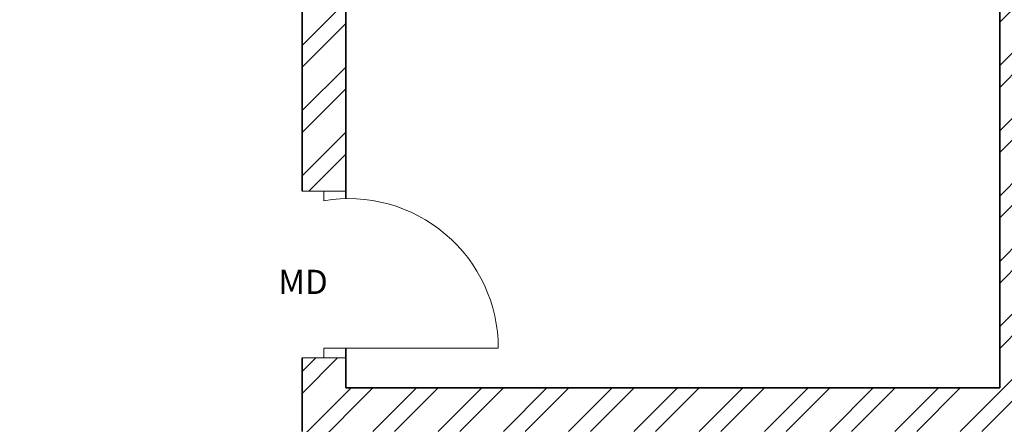
# Model space of a CAD drawing. Units: inches. Extents: x 2120 to 4013, y 1390 to 3019.
# Tile 35 of 59: x 2657 to 2861, y 1964 to 2048. Entities that reach past the tile are written whole.
import ezdxf

# ---------------------------------------------------------------- set-up
doc = ezdxf.new("R2010")
doc.units = ezdxf.units.IN
for name, color, linetype, lineweight in [('A-ANNO-TEXT', 7, 'Continuous', 18), ('A-DOOR', 3, 'Continuous', 18), ('A-WALL', 7, 'Continuous', 35), ('A-WALL-PATT', 252, 'Continuous', 13)]:
    doc.layers.add(name, color=color, linetype=linetype, lineweight=lineweight)
doc.styles.get("Standard").update_dxf_attribs({"font": 'arial.ttf'})

msp = doc.modelspace()

# ---------------------------------------------------------------- hatches: boundary and pattern name
at = {"layer": 'A-WALL-PATT'}
h = msp.add_hatch(dxfattribs=at)
h.set_pattern_fill('ANSI32', color=256)
h.paths.add_polyline_path([(2271.7331, 2343.531), (2283.3788, 2343.531), (2283.3788, 2348.031), (2283.3788, 2352.5306), (2262.7331, 2352.5306), (2262.7331, 2182.638), (2267.2331, 2182.638), (2271.7331, 2182.638), (2271.7331, 2219.031), (2391.7331, 2219.031), (2391.7331, 2214.189), (2393.9831, 2214.189), (2396.2331, 2214.189), (2396.2331, 2219.031), (2420.2331, 2219.031), (2420.2331, 2225.7535), (2417.2197, 2225.7535), (2415.7331, 2225.7535), (2415.7331, 2223.5306), (2271.7331, 2223.5306)])
h.paths.add_polyline_path([(2380.0942, 2352.5306), (2343.3788, 2352.5306), (2343.3788, 2343.531), (2363.2331, 2343.531), (2363.2331, 2288.8489), (2365.4831, 2288.8489), (2367.7331, 2288.8489), (2367.7331, 2343.531), (2380.0942, 2343.531)], flags=17)
h.paths.add_polyline_path([(2432.4339, 2352.5306), (2404.0943, 2352.5306), (2404.0943, 2343.531), (2415.7331, 2343.531), (2415.7331, 2264.0306), (2367.7331, 2264.0306), (2367.7331, 2266.4872), (2363.2331, 2266.4872), (2363.2331, 2259.531), (2367.7331, 2259.531), (2415.7331, 2259.531), (2415.7331, 2255.0658), (2420.2331, 2255.0658), (2420.2331, 2259.531), (2424.5717, 2259.531), (2424.5717, 2261.781), (2424.5717, 2264.0306), (2420.2331, 2264.0306), (2420.2331, 2343.531), (2432.4339, 2343.531)])
h.paths.add_polyline_path([(2508.9115, 2352.5306), (2456.4339, 2352.5306), (2456.4339, 2343.531), (2468.2331, 2343.531), (2468.2331, 2264.0306), (2448.0487, 2264.0306), (2448.0487, 2259.531), (2468.2331, 2259.531), (2468.2331, 2255.5496), (2472.7331, 2255.5496), (2472.7331, 2343.531), (2508.9115, 2343.531)])
h.paths.add_polyline_path([(2637.7331, 2352.5306), (2544.9116, 2352.5306), (2544.9116, 2343.531), (2589.7331, 2343.531), (2633.2331, 2343.531), (2637.7331, 2343.531)])
h.paths.add_polyline_path([(2594.2331, 2343.5306), (2589.7331, 2343.5306), (2589.7331, 2259.5306), (2589.7331, 2252.4915), (2591.9831, 2252.4915), (2594.2331, 2252.4915)])
h.paths.add_polyline_path([(2637.7331, 2223.5306), (2594.2331, 2223.5306), (2594.2331, 2230.1988), (2591.9831, 2230.1988), (2589.7331, 2230.1988), (2589.7331, 2223.5306), (2472.7331, 2223.5306), (2468.2331, 2223.5306), (2468.2331, 2219.031), (2628.7331, 2219.031), (2628.7331, 2138.031), (2637.7331, 2138.031)])
h.paths.add_polyline_path([(3822.6535, 2458.4402), (3874.9468, 2458.4402), (3874.9468, 2476.9866), (3822.6535, 2476.9866)], flags=9)
h.paths.add_polyline_path([(3834.6921, 2781.8174), (3935.9206, 2781.8174), (3935.9206, 2800.3638), (3834.6921, 2800.3638)], flags=9)
h.paths.add_polyline_path([(3832.2843, 2837.9683), (3884.5776, 2837.9683), (3884.5776, 2856.5146), (3832.2843, 2856.5146)], flags=9)
h.paths.add_polyline_path([(3830.9388, 2861.4782), (3956.8958, 2861.4782), (3956.8958, 2880.0245), (3830.9388, 2880.0245)], flags=9)
h.paths.add_polyline_path([(3870.6966, 2352.5752), (3887.9272, 2352.5752), (3887.9272, 2377.3037), (3870.6966, 2377.3037)], flags=9)
h.paths.add_polyline_path([(3289.2701, 2413.161), (3435.2223, 2413.161), (3435.2223, 2450.2538), (3289.2701, 2450.2538)], flags=9)
h.paths.add_polyline_path([(2487.6944, 2414.3601), (2637.8335, 2414.3601), (2637.8335, 2451.4528), (2487.6944, 2451.4528)], flags=9)
h.paths.add_polyline_path([(2567.3724, 1457.9199), (2815.296, 1457.9199), (2815.296, 1495.0127), (2567.3724, 1495.0127)], flags=9)
h.paths.add_polyline_path([(2655.3825, 2093.2363), (2685.9555, 2093.2363), (2685.9555, 2111.8937), (2655.3825, 2111.8937)], flags=9)
h.paths.add_polyline_path([(2543.9218, 1550.6671), (2587.8406, 1550.6671), (2587.8406, 1569.3244), (2543.9218, 1569.3244)], flags=9)
h.paths.add_polyline_path([(2905.1384, 1543.8113), (2949.0572, 1543.8113), (2949.0572, 1562.4686), (2905.1384, 1562.4686)], flags=9)
h.paths.add_polyline_path([(2736.4118, 1702.4736), (2784.2153, 1702.4736), (2784.2153, 1721.1309), (2736.4118, 1721.1309)], flags=9)
h.paths.add_polyline_path([(2912.8666, 1710.4168), (2951.707, 1710.4168), (2951.707, 1729.0741), (2912.8666, 1729.0741)], flags=9)
h.paths.add_polyline_path([(2923.5785, 1763.5038), (2959.7279, 1763.5038), (2959.7279, 1782.1611), (2923.5785, 1782.1611)], flags=9)
h.paths.add_polyline_path([(2925.2114, 1809.6137), (2967.1861, 1809.6137), (2967.1861, 1828.271), (2925.2114, 1828.271)], flags=9)
h.paths.add_polyline_path([(2996.2711, 1878.9003), (2996.2711, 1913.109), (2977.6138, 1913.109), (2977.6138, 1878.9003)], flags=9)
h.paths.add_polyline_path([(2883.0859, 1895.7192), (2927.1855, 1895.7192), (2927.1855, 1914.3766), (2883.0859, 1914.3766)], flags=9)
h.paths.add_polyline_path([(2787.3924, 1810.8013), (2841.0213, 1810.8013), (2841.0213, 1829.4587), (2787.3924, 1829.4587)], flags=9)
h.paths.add_polyline_path([(2775.6399, 2101.7395), (2829.2689, 2101.7395), (2829.2689, 2120.3968), (2775.6399, 2120.3968)], flags=9)
h.paths.add_polyline_path([(2913.0263, 2075.817), (2951.8667, 2075.817), (2951.8667, 2094.4744), (2913.0263, 2094.4744)], flags=9)
h.paths.add_polyline_path([(2929.966, 2133.3669), (2966.1154, 2133.3669), (2966.1154, 2152.0243), (2929.966, 2152.0243)], flags=9)
h.paths.add_polyline_path([(2932.7502, 2182.6088), (2968.8996, 2182.6088), (2968.8996, 2201.2662), (2932.7502, 2201.2662)], flags=9)
h.paths.add_polyline_path([(2996.0681, 2266.3173), (2996.0681, 2300.5261), (2977.4108, 2300.5261), (2977.4108, 2266.3173)], flags=9)
h.paths.add_polyline_path([(2885.1039, 2279.2186), (2929.2035, 2279.2186), (2929.2035, 2297.8759), (2885.1039, 2297.8759)], flags=9)
h.paths.add_polyline_path([(2735.7042, 2218.3197), (2783.5078, 2218.3197), (2783.5078, 2236.9771), (2735.7042, 2236.9771)], flags=9)
h.paths.add_polyline_path([(2635.6049, 2044.0085), (2648.9678, 2044.0085), (2648.9678, 2054.312), (2635.6049, 2054.312)], flags=9)
h.paths.add_polyline_path([(2714.0148, 1923.0473), (2727.3777, 1923.0473), (2727.3777, 1933.3508), (2714.0148, 1933.3508)], flags=9)
h.paths.add_polyline_path([(2709.0345, 1988.1628), (2722.3974, 1988.1628), (2722.3974, 1998.4663), (2709.0345, 1998.4663)], flags=9)
h.paths.add_polyline_path([(2592.8935, 1962.1763), (2606.2564, 1962.1763), (2606.2564, 1972.4799), (2592.8935, 1972.4799)], flags=9)
h.paths.add_polyline_path([(2618.3996, 1985.9724), (2644.1942, 1985.9724), (2644.1942, 1996.2759), (2618.3996, 1996.2759)], flags=9)
h.paths.add_polyline_path([(2601.279, 1920.5869), (2614.6419, 1920.5869), (2614.6419, 1930.8904), (2601.279, 1930.8904)], flags=9)
h.paths.add_polyline_path([(2692.3278, 1932.7645), (2704.5311, 1932.7645), (2704.5311, 1943.0681), (2692.3278, 1943.0681)], flags=9)
h.paths.add_polyline_path([(2311.122, 1672.7318), (2355.0408, 1672.7318), (2355.0408, 1691.3892), (2311.122, 1691.3892)], flags=9)
h.paths.add_polyline_path([(2456.2551, 1632.3198), (2492.4796, 1632.3198), (2492.4796, 1650.9772), (2456.2551, 1650.9772)], flags=9)
h.paths.add_polyline_path([(2401.0766, 1631.4793), (2437.301, 1631.4793), (2437.301, 1650.1367), (2401.0766, 1650.1367)], flags=9)
h.paths.add_polyline_path([(2546.7054, 1700.9235), (2594.509, 1700.9235), (2594.509, 1719.5809), (2546.7054, 1719.5809)], flags=9)
h.paths.add_polyline_path([(2445.4866, 1766.9937), (2497.5261, 1766.9937), (2497.5261, 1785.651), (2445.4866, 1785.651)], flags=9)
h.paths.add_polyline_path([(2287.9992, 1739.7675), (2326.8396, 1739.7675), (2326.8396, 1758.4248), (2287.9992, 1758.4248)], flags=9)
h.paths.add_polyline_path([(2458.5279, 1924.7607), (2510.5675, 1924.7607), (2510.5675, 1943.4181), (2458.5279, 1943.4181)], flags=9)
h.paths.add_polyline_path([(2309.2811, 1902.7642), (2345.4305, 1902.7642), (2345.4305, 1921.4215), (2309.2811, 1921.4215)], flags=9)
h.paths.add_polyline_path([(2490.7554, 2018.9392), (2530.7896, 2018.9392), (2530.7896, 2037.5965), (2490.7554, 2037.5965)], flags=9)
h.paths.add_polyline_path([(2402.143, 2024.7393), (2438.5414, 2024.7393), (2438.5414, 2043.3966), (2402.143, 2043.3966)], flags=9)
h.paths.add_polyline_path([(2287.856, 1931.7926), (2326.6964, 1931.7926), (2326.6964, 1950.4499), (2287.856, 1950.4499)], flags=9)
h.paths.add_polyline_path([(2281.7979, 2193.5771), (2320.6383, 2193.5771), (2320.6383, 2212.2344), (2281.7979, 2212.2344)], flags=25)
h.paths.add_polyline_path([(2484.0754, 2093.892), (2536.115, 2093.892), (2536.115, 2112.5494), (2484.0754, 2112.5494)], flags=9)
h.paths.add_polyline_path([(2624.7948, 2281.8639), (2624.7948, 2311.4137), (2606.1375, 2311.4137), (2606.1375, 2281.8639)], flags=9)
h.paths.add_polyline_path([(2507.5036, 2290.3639), (2541.934, 2290.3639), (2541.934, 2309.0212), (2507.5036, 2309.0212)], flags=9)
h.paths.add_polyline_path([(2423.1076, 2285.2202), (2459.332, 2285.2202), (2459.332, 2303.8776), (2423.1076, 2303.8776)], flags=9)
h.paths.add_polyline_path([(2374.5467, 2289.6272), (2410.7711, 2289.6272), (2410.7711, 2308.2846), (2374.5467, 2308.2846)], flags=25)
h.paths.add_polyline_path([(2277.4907, 2227.5651), (2316.3311, 2227.5651), (2316.3311, 2246.2224), (2277.4907, 2246.2224)], flags=25)
h.paths.add_polyline_path([(2655.3825, 2093.2367), (2685.9555, 2093.2367), (2685.9555, 2111.894), (2655.3825, 2111.894)], flags=9)
h.paths.add_polyline_path([(2543.9217, 1550.6674), (2587.8406, 1550.6674), (2587.8406, 1569.3247), (2543.9217, 1569.3247)], flags=9)
h.paths.add_polyline_path([(2905.1384, 1543.8116), (2949.0572, 1543.8116), (2949.0572, 1562.4689), (2905.1384, 1562.4689)], flags=9)
h.paths.add_polyline_path([(2736.4118, 1702.4739), (2784.2153, 1702.4739), (2784.2153, 1721.1312), (2736.4118, 1721.1312)], flags=9)
h.paths.add_polyline_path([(2912.8666, 1710.4171), (2951.707, 1710.4171), (2951.707, 1729.0744), (2912.8666, 1729.0744)], flags=9)
h.paths.add_polyline_path([(2923.5785, 1763.5041), (2959.7279, 1763.5041), (2959.7279, 1782.1614), (2923.5785, 1782.1614)], flags=9)
h.paths.add_polyline_path([(2925.2114, 1809.614), (2967.1861, 1809.614), (2967.1861, 1828.2713), (2925.2114, 1828.2713)], flags=9)
h.paths.add_polyline_path([(2996.2711, 1878.9006), (2996.2711, 1913.1094), (2977.6137, 1913.1094), (2977.6137, 1878.9006)], flags=9)
h.paths.add_polyline_path([(2883.0859, 1895.7195), (2927.1855, 1895.7195), (2927.1855, 1914.3769), (2883.0859, 1914.3769)], flags=9)
h.paths.add_polyline_path([(2787.3924, 1810.8016), (2841.0213, 1810.8016), (2841.0213, 1829.459), (2787.3924, 1829.459)], flags=9)
h.paths.add_polyline_path([(2775.6399, 2101.7398), (2829.2688, 2101.7398), (2829.2688, 2120.3971), (2775.6399, 2120.3971)], flags=9)
h.paths.add_polyline_path([(2913.0263, 2075.8173), (2951.8667, 2075.8173), (2951.8667, 2094.4747), (2913.0263, 2094.4747)], flags=9)
h.paths.add_polyline_path([(2929.966, 2133.3672), (2966.1154, 2133.3672), (2966.1154, 2152.0246), (2929.966, 2152.0246)], flags=9)
h.paths.add_polyline_path([(2932.7502, 2182.6091), (2968.8996, 2182.6091), (2968.8996, 2201.2665), (2932.7502, 2201.2665)], flags=9)
h.paths.add_polyline_path([(2996.0681, 2266.3176), (2996.0681, 2300.5264), (2977.4108, 2300.5264), (2977.4108, 2266.3176)], flags=9)
h.paths.add_polyline_path([(2885.1039, 2279.2189), (2929.2035, 2279.2189), (2929.2035, 2297.8762), (2885.1039, 2297.8762)], flags=9)
h.paths.add_polyline_path([(2735.7042, 2218.32), (2783.5078, 2218.32), (2783.5078, 2236.9774), (2735.7042, 2236.9774)], flags=9)
h.paths.add_polyline_path([(2635.6048, 2044.0088), (2648.9677, 2044.0088), (2648.9677, 2054.3123), (2635.6048, 2054.3123)], flags=9)
h.paths.add_polyline_path([(2714.0148, 1923.0476), (2727.3777, 1923.0476), (2727.3777, 1933.3511), (2714.0148, 1933.3511)], flags=9)
h.paths.add_polyline_path([(2709.0345, 1988.1631), (2722.3974, 1988.1631), (2722.3974, 1998.4666), (2709.0345, 1998.4666)], flags=9)
h.paths.add_polyline_path([(2592.8935, 1962.1766), (2606.2564, 1962.1766), (2606.2564, 1972.4802), (2592.8935, 1972.4802)], flags=9)
h.paths.add_polyline_path([(2618.3995, 1985.9727), (2644.1942, 1985.9727), (2644.1942, 1996.2762), (2618.3995, 1996.2762)], flags=9)
h.paths.add_polyline_path([(2601.279, 1920.5872), (2614.6419, 1920.5872), (2614.6419, 1930.8908), (2601.279, 1930.8908)], flags=9)
h.paths.add_polyline_path([(2692.3278, 1932.7648), (2704.5311, 1932.7648), (2704.5311, 1943.0684), (2692.3278, 1943.0684)], flags=9)
h.paths.add_polyline_path([(2311.122, 1672.7321), (2355.0408, 1672.7321), (2355.0408, 1691.3895), (2311.122, 1691.3895)], flags=9)
h.paths.add_polyline_path([(2456.2551, 1632.3201), (2492.4795, 1632.3201), (2492.4795, 1650.9775), (2456.2551, 1650.9775)], flags=9)
h.paths.add_polyline_path([(2401.0766, 1631.4796), (2437.301, 1631.4796), (2437.301, 1650.137), (2401.0766, 1650.137)], flags=9)
h.paths.add_polyline_path([(2546.7054, 1700.9238), (2594.509, 1700.9238), (2594.509, 1719.5812), (2546.7054, 1719.5812)], flags=9)
h.paths.add_polyline_path([(2445.4866, 1766.994), (2497.5261, 1766.994), (2497.5261, 1785.6513), (2445.4866, 1785.6513)], flags=9)
h.paths.add_polyline_path([(2287.9992, 1739.7678), (2326.8396, 1739.7678), (2326.8396, 1758.4251), (2287.9992, 1758.4251)], flags=9)
h.paths.add_polyline_path([(2458.5279, 1924.7611), (2510.5675, 1924.7611), (2510.5675, 1943.4184), (2458.5279, 1943.4184)], flags=9)
h.paths.add_polyline_path([(2309.2811, 1902.7645), (2345.4305, 1902.7645), (2345.4305, 1921.4218), (2309.2811, 1921.4218)], flags=9)
h.paths.add_polyline_path([(2490.7554, 2018.9395), (2530.7895, 2018.9395), (2530.7895, 2037.5968), (2490.7554, 2037.5968)], flags=9)
h.paths.add_polyline_path([(2402.143, 2024.7396), (2438.5413, 2024.7396), (2438.5413, 2043.3969), (2402.143, 2043.3969)], flags=9)
h.paths.add_polyline_path([(2287.856, 1931.7929), (2326.6964, 1931.7929), (2326.6964, 1950.4502), (2287.856, 1950.4502)], flags=9)
h.paths.add_polyline_path([(2281.7979, 2193.5774), (2320.6383, 2193.5774), (2320.6383, 2212.2347), (2281.7979, 2212.2347)], flags=25)
h.paths.add_polyline_path([(2484.0754, 2093.8924), (2536.115, 2093.8924), (2536.115, 2112.5497), (2484.0754, 2112.5497)], flags=9)
h.paths.add_polyline_path([(2624.7948, 2281.8642), (2624.7948, 2311.414), (2606.1374, 2311.414), (2606.1374, 2281.8642)], flags=9)
h.paths.add_polyline_path([(2507.5035, 2290.3642), (2541.934, 2290.3642), (2541.934, 2309.0215), (2507.5035, 2309.0215)], flags=9)
h.paths.add_polyline_path([(2423.1075, 2285.2205), (2459.332, 2285.2205), (2459.332, 2303.8779), (2423.1075, 2303.8779)], flags=9)
h.paths.add_polyline_path([(2374.5467, 2289.6275), (2410.7711, 2289.6275), (2410.7711, 2308.2849), (2374.5467, 2308.2849)], flags=25)
h.paths.add_polyline_path([(2277.4907, 2227.5654), (2316.3311, 2227.5654), (2316.3311, 2246.2227), (2277.4907, 2246.2227)], flags=25)
h = msp.add_hatch(dxfattribs=at)
h.set_pattern_fill('ANSI32', color=256)
h.paths.add_polyline_path([(2271.7331, 1980.389), (2262.7331, 1980.389), (2262.7331, 1912.8434), (2267.2331, 1912.8434), (2271.7331, 1912.8434), (2271.7331, 1922.531), (2351.2331, 1922.531), (2351.2331, 1901.4728), (2355.7331, 1901.4728), (2355.7331, 1922.531), (2357.9815, 1922.531), (2357.9815, 1926.5306), (2271.7331, 1926.5306)])
h.paths.add_polyline_path([(2589.2331, 1949.1622), (2584.7331, 1949.1622), (2580.2331, 1949.1622), (2580.2331, 1874.5306), (2355.7331, 1874.5306), (2355.7331, 1880.1922), (2351.2331, 1880.1922), (2351.2331, 1874.5306), (2271.7331, 1874.5306), (2271.7331, 1888.8431), (2262.7331, 1888.8431), (2262.7331, 1842.2909), (2267.2331, 1842.2909), (2271.7331, 1842.2909), (2271.7331, 1865.531), (2415.7331, 1865.531), (2415.7331, 1779.7286), (2420.2331, 1779.7286), (2420.2331, 1865.531), (2589.2331, 1865.531)])
h.paths.add_polyline_path([(2271.7331, 1782.2906), (2262.7331, 1782.2906), (2262.7331, 1711.4639), (2267.2331, 1711.4639), (2271.7331, 1711.4639), (2271.7331, 1738.031), (2420.2331, 1738.031), (2420.2331, 1742.531), (2420.2331, 1747.3376), (2417.9831, 1747.3376), (2415.7331, 1747.3376), (2415.7331, 1742.5306), (2271.7331, 1742.5306)])
h.paths.add_polyline_path([(2271.7331, 1627.031), (2362.3957, 1627.031), (2362.3957, 1629.281), (2362.3957, 1631.5306), (2271.7331, 1631.5306), (2271.7331, 1675.4636), (2262.7331, 1675.4636), (2262.7331, 1581.531), (2405.3032, 1581.531), (2405.3032, 1586.031), (2405.3032, 1590.5306), (2396.2331, 1590.5306), (2396.2331, 1691.4513), (2418.7206, 1691.4513), (2418.7206, 1695.951), (2396.2331, 1695.951), (2391.7331, 1695.951), (2391.7331, 1631.5306), (2386.7425, 1631.5306), (2386.7425, 1629.2806), (2386.7425, 1627.031), (2391.7331, 1627.031), (2391.7331, 1586.1709), (2271.7331, 1586.1709)])
h.paths.add_polyline_path([(2459.6703, 1590.5306), (2429.3032, 1590.5306), (2429.3032, 1581.531), (2459.6703, 1581.531), (2459.6703, 1586.031)])
h.paths.add_polyline_path([(2501.2331, 1590.531), (2501.2331, 1665.0195), (2498.9831, 1665.0195), (2496.7331, 1665.0195), (2496.7331, 1590.5306), (2483.8201, 1590.5306), (2483.8201, 1590.1579), (2483.6704, 1590.1579), (2483.6704, 1581.531), (2505.0196, 1581.531), (2505.0196, 1583.781), (2505.0196, 1586.0306), (2501.2331, 1586.0306)])
h.paths.add_polyline_path([(2544.1361, 1583.781), (2544.1361, 1586.0306), (2527.1368, 1586.0306), (2527.1368, 1583.7806), (2527.1368, 1581.531), (2544.1361, 1581.531)])
h.paths.add_polyline_path([(3822.6535, 2458.4402), (3874.9468, 2458.4402), (3874.9468, 2476.9866), (3822.6535, 2476.9866)], flags=9)
h.paths.add_polyline_path([(3834.6921, 2781.8174), (3935.9206, 2781.8174), (3935.9206, 2800.3638), (3834.6921, 2800.3638)], flags=9)
h.paths.add_polyline_path([(3832.2843, 2837.9683), (3884.5776, 2837.9683), (3884.5776, 2856.5146), (3832.2843, 2856.5146)], flags=9)
h.paths.add_polyline_path([(3830.9388, 2861.4782), (3956.8958, 2861.4782), (3956.8958, 2880.0245), (3830.9388, 2880.0245)], flags=9)
h.paths.add_polyline_path([(3870.6966, 2352.5752), (3887.9272, 2352.5752), (3887.9272, 2377.3037), (3870.6966, 2377.3037)], flags=9)
h.paths.add_polyline_path([(3289.2701, 2413.161), (3435.2223, 2413.161), (3435.2223, 2450.2538), (3289.2701, 2450.2538)], flags=9)
h.paths.add_polyline_path([(2487.6944, 2414.3601), (2637.8335, 2414.3601), (2637.8335, 2451.4528), (2487.6944, 2451.4528)], flags=9)
h.paths.add_polyline_path([(2567.3724, 1457.9199), (2815.296, 1457.9199), (2815.296, 1495.0127), (2567.3724, 1495.0127)], flags=9)
h.paths.add_polyline_path([(2655.3825, 2093.2363), (2685.9555, 2093.2363), (2685.9555, 2111.8937), (2655.3825, 2111.8937)], flags=9)
h.paths.add_polyline_path([(2543.9218, 1550.6671), (2587.8406, 1550.6671), (2587.8406, 1569.3244), (2543.9218, 1569.3244)], flags=9)
h.paths.add_polyline_path([(2905.1384, 1543.8113), (2949.0572, 1543.8113), (2949.0572, 1562.4686), (2905.1384, 1562.4686)], flags=9)
h.paths.add_polyline_path([(2736.4118, 1702.4736), (2784.2153, 1702.4736), (2784.2153, 1721.1309), (2736.4118, 1721.1309)], flags=9)
h.paths.add_polyline_path([(2912.8666, 1710.4168), (2951.707, 1710.4168), (2951.707, 1729.0741), (2912.8666, 1729.0741)], flags=9)
h.paths.add_polyline_path([(2923.5785, 1763.5038), (2959.7279, 1763.5038), (2959.7279, 1782.1611), (2923.5785, 1782.1611)], flags=9)
h.paths.add_polyline_path([(2925.2114, 1809.6137), (2967.1861, 1809.6137), (2967.1861, 1828.271), (2925.2114, 1828.271)], flags=9)
h.paths.add_polyline_path([(2996.2711, 1878.9003), (2996.2711, 1913.109), (2977.6138, 1913.109), (2977.6138, 1878.9003)], flags=9)
h.paths.add_polyline_path([(2883.0859, 1895.7192), (2927.1855, 1895.7192), (2927.1855, 1914.3766), (2883.0859, 1914.3766)], flags=9)
h.paths.add_polyline_path([(2787.3924, 1810.8013), (2841.0213, 1810.8013), (2841.0213, 1829.4587), (2787.3924, 1829.4587)], flags=9)
h.paths.add_polyline_path([(2775.6399, 2101.7395), (2829.2689, 2101.7395), (2829.2689, 2120.3968), (2775.6399, 2120.3968)], flags=9)
h.paths.add_polyline_path([(2913.0263, 2075.817), (2951.8667, 2075.817), (2951.8667, 2094.4744), (2913.0263, 2094.4744)], flags=9)
h.paths.add_polyline_path([(2929.966, 2133.3669), (2966.1154, 2133.3669), (2966.1154, 2152.0243), (2929.966, 2152.0243)], flags=9)
h.paths.add_polyline_path([(2932.7502, 2182.6088), (2968.8996, 2182.6088), (2968.8996, 2201.2662), (2932.7502, 2201.2662)], flags=9)
h.paths.add_polyline_path([(2996.0681, 2266.3173), (2996.0681, 2300.5261), (2977.4108, 2300.5261), (2977.4108, 2266.3173)], flags=9)
h.paths.add_polyline_path([(2885.1039, 2279.2186), (2929.2035, 2279.2186), (2929.2035, 2297.8759), (2885.1039, 2297.8759)], flags=9)
h.paths.add_polyline_path([(2735.7042, 2218.3197), (2783.5078, 2218.3197), (2783.5078, 2236.9771), (2735.7042, 2236.9771)], flags=9)
h.paths.add_polyline_path([(2635.6049, 2044.0085), (2648.9678, 2044.0085), (2648.9678, 2054.312), (2635.6049, 2054.312)], flags=9)
h.paths.add_polyline_path([(2714.0148, 1923.0473), (2727.3777, 1923.0473), (2727.3777, 1933.3508), (2714.0148, 1933.3508)], flags=9)
h.paths.add_polyline_path([(2709.0345, 1988.1628), (2722.3974, 1988.1628), (2722.3974, 1998.4663), (2709.0345, 1998.4663)], flags=9)
h.paths.add_polyline_path([(2592.8935, 1962.1763), (2606.2564, 1962.1763), (2606.2564, 1972.4799), (2592.8935, 1972.4799)], flags=9)
h.paths.add_polyline_path([(2618.3996, 1985.9724), (2644.1942, 1985.9724), (2644.1942, 1996.2759), (2618.3996, 1996.2759)], flags=9)
h.paths.add_polyline_path([(2601.279, 1920.5869), (2614.6419, 1920.5869), (2614.6419, 1930.8904), (2601.279, 1930.8904)], flags=9)
h.paths.add_polyline_path([(2692.3278, 1932.7645), (2704.5311, 1932.7645), (2704.5311, 1943.0681), (2692.3278, 1943.0681)], flags=9)
h.paths.add_polyline_path([(2311.122, 1672.7318), (2355.0408, 1672.7318), (2355.0408, 1691.3892), (2311.122, 1691.3892)], flags=25)
h.paths.add_polyline_path([(2456.2551, 1632.3198), (2492.4796, 1632.3198), (2492.4796, 1650.9772), (2456.2551, 1650.9772)], flags=9)
h.paths.add_polyline_path([(2401.0766, 1631.4793), (2437.301, 1631.4793), (2437.301, 1650.1367), (2401.0766, 1650.1367)], flags=9)
h.paths.add_polyline_path([(2546.7054, 1700.9235), (2594.509, 1700.9235), (2594.509, 1719.5809), (2546.7054, 1719.5809)], flags=9)
h.paths.add_polyline_path([(2445.4866, 1766.9937), (2497.5261, 1766.9937), (2497.5261, 1785.651), (2445.4866, 1785.651)], flags=9)
h.paths.add_polyline_path([(2287.9992, 1739.7675), (2326.8396, 1739.7675), (2326.8396, 1758.4248), (2287.9992, 1758.4248)], flags=24)
h.paths.add_polyline_path([(2458.5279, 1924.7607), (2510.5675, 1924.7607), (2510.5675, 1943.4181), (2458.5279, 1943.4181)], flags=25)
h.paths.add_polyline_path([(2309.2811, 1902.7642), (2345.4305, 1902.7642), (2345.4305, 1921.4215), (2309.2811, 1921.4215)], flags=25)
h.paths.add_polyline_path([(2490.7554, 2018.9392), (2530.7896, 2018.9392), (2530.7896, 2037.5965), (2490.7554, 2037.5965)], flags=9)
h.paths.add_polyline_path([(2402.143, 2024.7393), (2438.5414, 2024.7393), (2438.5414, 2043.3966), (2402.143, 2043.3966)], flags=9)
h.paths.add_polyline_path([(2287.856, 1931.7926), (2326.6964, 1931.7926), (2326.6964, 1950.4499), (2287.856, 1950.4499)], flags=25)
h.paths.add_polyline_path([(2281.7979, 2193.5771), (2320.6383, 2193.5771), (2320.6383, 2212.2344), (2281.7979, 2212.2344)], flags=9)
h.paths.add_polyline_path([(2484.0754, 2093.892), (2536.115, 2093.892), (2536.115, 2112.5494), (2484.0754, 2112.5494)], flags=9)
h.paths.add_polyline_path([(2624.7948, 2281.8639), (2624.7948, 2311.4137), (2606.1375, 2311.4137), (2606.1375, 2281.8639)], flags=9)
h.paths.add_polyline_path([(2507.5036, 2290.3639), (2541.934, 2290.3639), (2541.934, 2309.0212), (2507.5036, 2309.0212)], flags=9)
h.paths.add_polyline_path([(2423.1076, 2285.2202), (2459.332, 2285.2202), (2459.332, 2303.8776), (2423.1076, 2303.8776)], flags=9)
h.paths.add_polyline_path([(2374.5467, 2289.6272), (2410.7711, 2289.6272), (2410.7711, 2308.2846), (2374.5467, 2308.2846)], flags=9)
h.paths.add_polyline_path([(2277.4907, 2227.5651), (2316.3311, 2227.5651), (2316.3311, 2246.2224), (2277.4907, 2246.2224)], flags=9)
h.paths.add_polyline_path([(2655.3825, 2093.2367), (2685.9555, 2093.2367), (2685.9555, 2111.894), (2655.3825, 2111.894)], flags=9)
h.paths.add_polyline_path([(2543.9217, 1550.6674), (2587.8406, 1550.6674), (2587.8406, 1569.3247), (2543.9217, 1569.3247)], flags=9)
h.paths.add_polyline_path([(2905.1384, 1543.8116), (2949.0572, 1543.8116), (2949.0572, 1562.4689), (2905.1384, 1562.4689)], flags=9)
h.paths.add_polyline_path([(2736.4118, 1702.4739), (2784.2153, 1702.4739), (2784.2153, 1721.1312), (2736.4118, 1721.1312)], flags=9)
h.paths.add_polyline_path([(2912.8666, 1710.4171), (2951.707, 1710.4171), (2951.707, 1729.0744), (2912.8666, 1729.0744)], flags=9)
h.paths.add_polyline_path([(2923.5785, 1763.5041), (2959.7279, 1763.5041), (2959.7279, 1782.1614), (2923.5785, 1782.1614)], flags=9)
h.paths.add_polyline_path([(2925.2114, 1809.614), (2967.1861, 1809.614), (2967.1861, 1828.2713), (2925.2114, 1828.2713)], flags=9)
h.paths.add_polyline_path([(2996.2711, 1878.9006), (2996.2711, 1913.1094), (2977.6137, 1913.1094), (2977.6137, 1878.9006)], flags=9)
h.paths.add_polyline_path([(2883.0859, 1895.7195), (2927.1855, 1895.7195), (2927.1855, 1914.3769), (2883.0859, 1914.3769)], flags=9)
h.paths.add_polyline_path([(2787.3924, 1810.8016), (2841.0213, 1810.8016), (2841.0213, 1829.459), (2787.3924, 1829.459)], flags=9)
h.paths.add_polyline_path([(2775.6399, 2101.7398), (2829.2688, 2101.7398), (2829.2688, 2120.3971), (2775.6399, 2120.3971)], flags=9)
h.paths.add_polyline_path([(2913.0263, 2075.8173), (2951.8667, 2075.8173), (2951.8667, 2094.4747), (2913.0263, 2094.4747)], flags=9)
h.paths.add_polyline_path([(2929.966, 2133.3672), (2966.1154, 2133.3672), (2966.1154, 2152.0246), (2929.966, 2152.0246)], flags=9)
h.paths.add_polyline_path([(2932.7502, 2182.6091), (2968.8996, 2182.6091), (2968.8996, 2201.2665), (2932.7502, 2201.2665)], flags=9)
h.paths.add_polyline_path([(2996.0681, 2266.3176), (2996.0681, 2300.5264), (2977.4108, 2300.5264), (2977.4108, 2266.3176)], flags=9)
h.paths.add_polyline_path([(2885.1039, 2279.2189), (2929.2035, 2279.2189), (2929.2035, 2297.8762), (2885.1039, 2297.8762)], flags=9)
h.paths.add_polyline_path([(2735.7042, 2218.32), (2783.5078, 2218.32), (2783.5078, 2236.9774), (2735.7042, 2236.9774)], flags=9)
h.paths.add_polyline_path([(2635.6048, 2044.0088), (2648.9677, 2044.0088), (2648.9677, 2054.3123), (2635.6048, 2054.3123)], flags=9)
h.paths.add_polyline_path([(2714.0148, 1923.0476), (2727.3777, 1923.0476), (2727.3777, 1933.3511), (2714.0148, 1933.3511)], flags=9)
h.paths.add_polyline_path([(2709.0345, 1988.1631), (2722.3974, 1988.1631), (2722.3974, 1998.4666), (2709.0345, 1998.4666)], flags=9)
h.paths.add_polyline_path([(2592.8935, 1962.1766), (2606.2564, 1962.1766), (2606.2564, 1972.4802), (2592.8935, 1972.4802)], flags=9)
h.paths.add_polyline_path([(2618.3995, 1985.9727), (2644.1942, 1985.9727), (2644.1942, 1996.2762), (2618.3995, 1996.2762)], flags=9)
h.paths.add_polyline_path([(2601.279, 1920.5872), (2614.6419, 1920.5872), (2614.6419, 1930.8908), (2601.279, 1930.8908)], flags=9)
h.paths.add_polyline_path([(2692.3278, 1932.7648), (2704.5311, 1932.7648), (2704.5311, 1943.0684), (2692.3278, 1943.0684)], flags=9)
h.paths.add_polyline_path([(2311.122, 1672.7321), (2355.0408, 1672.7321), (2355.0408, 1691.3895), (2311.122, 1691.3895)], flags=25)
h.paths.add_polyline_path([(2456.2551, 1632.3201), (2492.4795, 1632.3201), (2492.4795, 1650.9775), (2456.2551, 1650.9775)], flags=9)
h.paths.add_polyline_path([(2401.0766, 1631.4796), (2437.301, 1631.4796), (2437.301, 1650.137), (2401.0766, 1650.137)], flags=9)
h.paths.add_polyline_path([(2546.7054, 1700.9238), (2594.509, 1700.9238), (2594.509, 1719.5812), (2546.7054, 1719.5812)], flags=9)
h.paths.add_polyline_path([(2445.4866, 1766.994), (2497.5261, 1766.994), (2497.5261, 1785.6513), (2445.4866, 1785.6513)], flags=9)
h.paths.add_polyline_path([(2287.9992, 1739.7678), (2326.8396, 1739.7678), (2326.8396, 1758.4251), (2287.9992, 1758.4251)], flags=24)
h.paths.add_polyline_path([(2458.5279, 1924.7611), (2510.5675, 1924.7611), (2510.5675, 1943.4184), (2458.5279, 1943.4184)], flags=25)
h.paths.add_polyline_path([(2309.2811, 1902.7645), (2345.4305, 1902.7645), (2345.4305, 1921.4218), (2309.2811, 1921.4218)], flags=25)
h.paths.add_polyline_path([(2490.7554, 2018.9395), (2530.7895, 2018.9395), (2530.7895, 2037.5968), (2490.7554, 2037.5968)], flags=9)
h.paths.add_polyline_path([(2402.143, 2024.7396), (2438.5413, 2024.7396), (2438.5413, 2043.3969), (2402.143, 2043.3969)], flags=9)
h.paths.add_polyline_path([(2287.856, 1931.7929), (2326.6964, 1931.7929), (2326.6964, 1950.4502), (2287.856, 1950.4502)], flags=25)
h.paths.add_polyline_path([(2281.7979, 2193.5774), (2320.6383, 2193.5774), (2320.6383, 2212.2347), (2281.7979, 2212.2347)], flags=9)
h.paths.add_polyline_path([(2484.0754, 2093.8924), (2536.115, 2093.8924), (2536.115, 2112.5497), (2484.0754, 2112.5497)], flags=9)
h.paths.add_polyline_path([(2624.7948, 2281.8642), (2624.7948, 2311.414), (2606.1374, 2311.414), (2606.1374, 2281.8642)], flags=9)
h.paths.add_polyline_path([(2507.5035, 2290.3642), (2541.934, 2290.3642), (2541.934, 2309.0215), (2507.5035, 2309.0215)], flags=9)
h.paths.add_polyline_path([(2423.1075, 2285.2205), (2459.332, 2285.2205), (2459.332, 2303.8779), (2423.1075, 2303.8779)], flags=9)
h.paths.add_polyline_path([(2374.5467, 2289.6275), (2410.7711, 2289.6275), (2410.7711, 2308.2849), (2374.5467, 2308.2849)], flags=9)
h.paths.add_polyline_path([(2277.4907, 2227.5654), (2316.3311, 2227.5654), (2316.3311, 2246.2227), (2277.4907, 2246.2227)], flags=9)
h = msp.add_hatch(dxfattribs=at)
h.set_pattern_fill('ANSI32', color=256)
h.paths.add_polyline_path([(2271.7331, 2122.6377), (2262.7331, 2122.6377), (2262.7331, 2040.3893), (2267.2331, 2040.3893), (2271.7331, 2040.3893), (2271.7331, 2044.8856), (2271.7331, 2070.531), (2391.7331, 2070.531), (2391.7331, 1926.5306), (2388.3993, 1926.5306), (2388.3993, 1922.531), (2395.7331, 1922.531), (2395.7331, 1992.531), (2400.4511, 1992.531), (2400.4511, 1997.0306), (2395.7331, 1997.0306), (2395.7331, 2070.531), (2443.7331, 2070.531), (2443.7331, 2046.1368), (2448.2331, 2046.1368), (2448.2331, 2070.531), (2580.2331, 2070.531), (2580.2331, 1997.0306), (2492.9076, 1997.0306), (2492.9076, 1992.531), (2580.2331, 1992.531), (2580.2331, 1983.9368), (2589.2331, 1983.9368), (2589.2331, 2070.531), (2589.2331, 2075.0306), (2396.2331, 2075.0306), (2396.2331, 2184.3565), (2393.9831, 2184.3565), (2391.7331, 2184.3565), (2391.7331, 2075.0306), (2271.7331, 2075.0306)])
h.paths.add_polyline_path([(2724.7331, 2138.0306), (2628.7331, 2138.0306), (2628.7331, 2070.5306), (2628.7331, 2067.0987), (2633.2331, 2067.0987), (2637.7331, 2067.0987), (2637.7331, 2070.531), (2657.3413, 2070.531), (2657.3413, 2079.5306), (2637.7331, 2079.5306), (2637.7331, 2129.031), (2715.7331, 2129.031), (2715.7331, 2079.5306), (2698.0378, 2079.5306), (2698.0378, 2070.531), (2715.7331, 2070.531), (2715.7331, 2012.1531), (2720.2331, 2012.1531), (2724.7331, 2012.1531)])
h.paths.add_polyline_path([(2724.7331, 2213.031), (2831.3209, 2213.031), (2831.3209, 2215.281), (2831.3209, 2217.5306), (2724.7331, 2217.5306), (2724.7331, 2343.531), (2751.8755, 2343.531), (2751.8755, 2352.5306), (2715.7331, 2352.5306), (2715.7331, 2138.031), (2724.7331, 2138.031)])
h.paths.add_polyline_path([(2902.53, 2352.5306), (2811.8755, 2352.5306), (2811.8755, 2343.531), (2867.2331, 2343.531), (2867.2331, 2217.5306), (2863.6364, 2217.5306), (2863.6364, 2213.031), (2871.7331, 2213.031), (2871.7331, 2217.531), (2871.7331, 2343.531), (2902.53, 2343.531)])
h.paths.add_polyline_path([(3009.7331, 2352.5306), (2938.53, 2352.5306), (2938.53, 2343.531), (2966.2331, 2343.531), (2966.2331, 2242.3281), (2968.4831, 2242.3281), (2970.7331, 2242.3281), (2970.7331, 2343.531), (3009.7331, 2343.531)])
h.paths.add_polyline_path([(3009.7331, 2217.5306), (2970.7331, 2217.5306), (2970.7331, 2220.5422), (2968.4831, 2220.5422), (2966.2331, 2220.5422), (2966.2331, 2217.5306), (2911.7752, 2217.5306), (2907.7331, 2217.5306), (2907.7331, 2213.0306), (2907.7331, 2194.9663), (2912.2331, 2194.9663), (2912.2331, 2213.031), (2970.7331, 2213.031), (3000.7331, 2213.031), (3000.7331, 2205.523), (3009.7331, 2205.523)])
h.paths.add_polyline_path([(3009.7331, 2181.5227), (3000.7331, 2181.5227), (3000.7331, 2165.0306), (2912.2331, 2165.0306), (2912.2331, 2170.8202), (2907.7331, 2170.8202), (2907.7331, 2165.0306), (2899.5169, 2165.0306), (2899.5169, 2162.7806), (2899.5169, 2160.531), (2907.7331, 2160.531), (2907.7331, 2137.3432), (2912.2331, 2137.3432), (2912.2331, 2160.531), (3000.7331, 2160.531), (3000.7331, 2150.4993), (3009.7331, 2150.4993)])
h.paths.add_polyline_path([(3009.7331, 2126.499), (3005.2331, 2126.499), (3000.7331, 2126.499), (3000.7331, 2112.5306), (2912.2331, 2112.5306), (2912.2331, 2115.6036), (2907.7331, 2115.6036), (2907.7331, 2108.031), (3000.7331, 2108.031), (3000.7331, 2084.7256), (3009.7331, 2084.7256)], flags=17)
h.paths.add_polyline_path([(3009.7331, 1971.531), (3009.7331, 2024.7253), (3000.7331, 2024.7253), (3000.7331, 2006.4153), (3000.7331, 1971.5306), (2864.2331, 1971.5306), (2864.2331, 2160.531), (2868.0522, 2160.531), (2868.0522, 2165.0306), (2859.7331, 2165.0306), (2859.7331, 1971.5306), (2724.7331, 1971.5306), (2724.7331, 1977.7012), (2715.7331, 1977.7012), (2715.7331, 1962.5306), (2715.7331, 1950.9035), (2720.2331, 1950.9035), (2724.7331, 1950.9035), (2724.7331, 1962.531), (2855.2331, 1962.531), (2859.7331, 1962.531), (2859.7331, 1835.031), (2864.2331, 1834.8158), (2864.2331, 1962.531), (2958.7331, 1962.531), (2958.7331, 1937.0925), (2963.2331, 1937.0925), (2963.2331, 1962.531), (3000.7331, 1962.531), (3009.7331, 1962.531)])
h.paths.add_polyline_path([(2724.7331, 1728.531), (2822.7164, 1728.531), (2822.7164, 1733.0306), (2724.7331, 1733.0306), (2724.7331, 1779.3416), (2715.7331, 1779.3416), (2715.7331, 1581.531), (2753.02, 1581.531), (2753.02, 1586.031), (2753.02, 1590.5306), (2724.7331, 1590.5306)])
h.paths.add_polyline_path([(2864.2331, 1590.531), (2864.2331, 1787.031), (2868.4075, 1787.031), (2868.4075, 1791.5306), (2859.7331, 1791.5306), (2859.7331, 1739.0306), (2859.7331, 1733.0306), (2854.3125, 1733.0306), (2854.3125, 1728.531), (2859.7331, 1728.531), (2859.7331, 1590.5306), (2813.02, 1590.5306), (2813.02, 1581.531), (2868.4123, 1581.531), (2868.4123, 1583.781), (2868.4123, 1586.0306), (2864.2331, 1586.0306)])
h.paths.add_polyline_path([(3009.7331, 1754.6619), (3000.7331, 1754.6619), (3000.7331, 1739.0306), (2912.2331, 1739.0306), (2912.2331, 1742.2257), (2907.7331, 1742.2257), (2907.7331, 1739.0306), (2907.7331, 1734.531), (3000.7331, 1734.531), (3000.7331, 1590.5306), (3000.7331, 1586.0306), (2971.3921, 1586.0306), (2971.3921, 1581.531), (3009.7331, 1581.531)])
h.paths.add_polyline_path([(2911.3921, 1583.781), (2911.3921, 1586.0306), (2891.2138, 1586.0306), (2891.2138, 1581.531), (2911.3921, 1581.531)])
h.paths.add_polyline_path([(3009.7331, 1799.8422), (3000.7331, 1799.8422), (3000.7331, 1791.5306), (2912.2331, 1791.5306), (2912.2331, 1796.3264), (2909.9831, 1796.3264), (2907.7331, 1796.3264), (2907.7331, 1791.5306), (2902.7033, 1791.5306), (2902.7033, 1787.031), (2907.7331, 1787.031), (2907.7331, 1761.1622), (2912.2331, 1761.1622), (2912.2331, 1787.031), (3000.7331, 1787.031), (3000.7331, 1778.6622), (3009.7331, 1778.6622)])
h.paths.add_polyline_path([(3009.7331, 1839.5306), (2963.2331, 1839.5306), (2963.2331, 1842.8629), (2960.9831, 1842.8629), (2958.7331, 1842.8629), (2958.7331, 1839.5306), (2907.7331, 1839.5306), (2907.7331, 1814.4599), (2912.2331, 1814.4599), (2912.2331, 1835.031), (3000.7331, 1835.031), (3000.7331, 1823.8425), (3009.7331, 1823.8425), (3009.7331, 1835.031)])
h.paths.add_polyline_path([(2963.2331, 1901.0922), (2960.9831, 1901.0922), (2958.7331, 1901.0922), (2958.7331, 1862.8843), (2963.2331, 1862.8843)], flags=17)
h.paths.add_polyline_path([(2724.7331, 1891.9826), (2724.7331, 1914.3416), (2715.7331, 1914.3416), (2715.7331, 1783.8416), (2637.7331, 1783.8416), (2637.7331, 1914.3416), (2628.7331, 1914.3416), (2624.7701, 1914.3416), (2624.7701, 1909.8416), (2624.7701, 1905.3419), (2628.7331, 1905.3419), (2628.7331, 1876.9915), (2628.7331, 1779.3419), (2637.7331, 1779.3419), (2715.7331, 1779.3419), (2724.7331, 1779.3419), (2724.7331, 1835.031)])
h.paths.add_polyline_path([(2637.7331, 1731.531), (2637.7331, 1779.3416), (2628.7331, 1779.3416), (2628.7331, 1731.5306), (2589.2331, 1731.5306), (2535.9814, 1731.5306), (2496.7331, 1731.5306), (2496.7331, 1725.6876), (2498.9831, 1725.6876), (2501.2331, 1725.6876), (2501.2331, 1727.031), (2628.7331, 1727.031), (2628.7331, 1680.4203), (2628.7331, 1590.5306), (2628.7331, 1586.0306), (2604.1361, 1586.0306), (2604.1361, 1581.531), (2637.7331, 1581.531), (2637.7331, 1590.531)])

# ---------------------------------------------------------------- linework, layer by layer
at = {"layer": 'A-DOOR'}
for p, q in [((2724.7331, 2012.1531), (2715.7331, 2012.1531)), ((2715.7331, 2012.1531), (2720.2331, 2012.1531)), ((2724.7331, 2012.1528), (2715.7331, 2012.1528)), ((2715.7331, 2012.1528), (2720.2331, 2012.1528)), ((2720.2331, 2012.1531), (2720.2331, 2010.1531)), ((2720.2331, 2012.1528), (2720.2331, 2010.1528)), ((2720.2331, 1977.7015), (2720.2331, 1979.7015)), ((2720.2331, 1979.7015), (2756.2331, 1979.7015)), ((2720.2331, 1977.7012), (2720.2331, 1979.7012)), ((2720.2331, 1979.7012), (2756.2331, 1979.7012)), ((2724.7331, 1977.7015), (2715.7331, 1977.7015)), ((2715.7331, 1977.7015), (2720.2331, 1977.7015)), ((2724.7331, 1977.7012), (2715.7331, 1977.7012)), ((2715.7331, 1977.7012), (2720.2331, 1977.7012))]:
    msp.add_line(p, q, dxfattribs=at)
for centre in [(2725.3539, 1979.7015), (2725.354, 1979.7012)]:
    msp.add_arc(centre, 30.8792, 360, 99.545687, dxfattribs=at)
at = {"layer": 'A-WALL'}
for p, q in [((2724.7331, 2213.031), (2724.7331, 2010.5745)), ((2724.7331, 2213.0306), (2724.7331, 2010.5742)), ((2859.7331, 1971.531), (2859.7331, 2165.031)), ((2859.7331, 1971.5306), (2859.7331, 2165.0306)), ((2715.7331, 2070.531), (2715.7331, 2012.1531)), ((2715.7331, 2070.5306), (2715.7331, 2012.1528)), ((2724.7331, 1979.7015), (2724.7331, 1971.531)), ((2724.7331, 1979.7012), (2724.7331, 1971.5306)), ((2715.7331, 1977.7015), (2715.7331, 1962.531)), ((2715.7331, 1977.7012), (2715.7331, 1962.5306)), ((2724.7331, 1971.531), (2859.7331, 1971.531)), ((2724.7331, 1971.5306), (2859.7331, 1971.5306))]:
    msp.add_line(p, q, dxfattribs=at)

# ---------------------------------------------------------------- texts
at = {"layer": 'A-ANNO-TEXT', "char_height": 5, "attachment_point": 1}
for insert in [(2710.8029, 1995.8933), (2710.8029, 1995.893)]:
    msp.add_mtext_dynamic_manual_height_columns('MD', width=56.213303, gutter_width=12.5, heights=[0], dxfattribs=dict(at, insert=insert))

doc.saveas('drawing.dxf')
